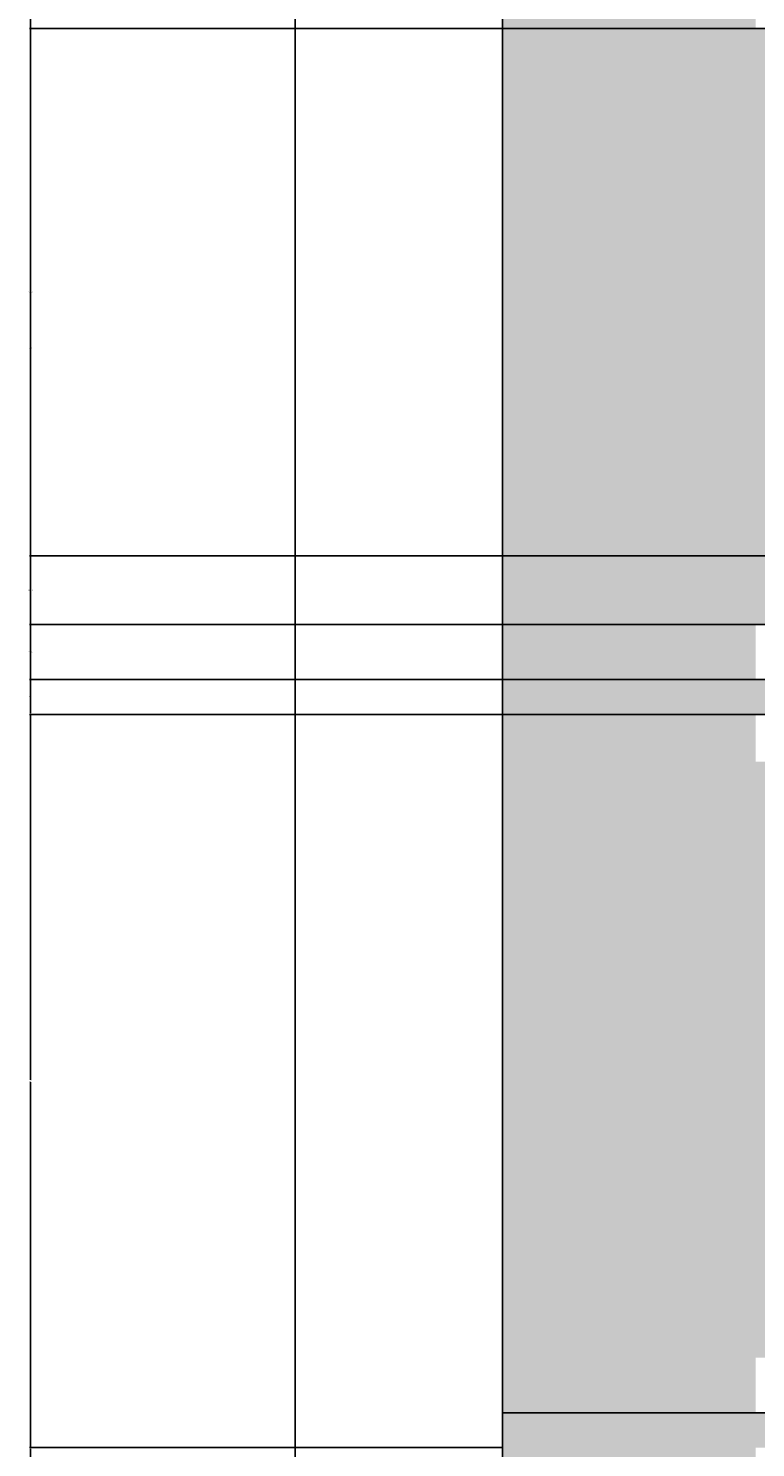
# Model space of a CAD drawing. Units: inches. Extents: x 3024 to 4744, y 1110 to 2100.
# Tile 18 of 29: x 3024 to 3149, y 1654 to 1897. Entities that reach past the tile are written whole.
import ezdxf

# ---------------------------------------------------------------- set-up
doc = ezdxf.new("R2010")
doc.units = ezdxf.units.IN
for name, color, linetype, lineweight in [('A-ANNO-DIMS', 2, 'Continuous', 18), ('A-ELEV', 7, 'Continuous', 25), ('A-ELEV-PATT', 252, 'Continuous', 13)]:
    doc.layers.add(name, color=color, linetype=linetype, lineweight=lineweight)
doc.styles.get("Standard").update_dxf_attribs({"font": 'arial.ttf'})
doc.dimstyles.get("Standard").update_dxf_attribs({"dimtxt": 0.18, "dimasz": 0.18, "dimexe": 0.18, "dimexo": 0.0625, "dimgap": 0.09, "dimtad": 0, "dimtih": 1, "dimtoh": 1, "dimdec": 1, "dimzin": 0, "dimdsep": 46, "dimlunit": 3, "dimtxsty": 'Standard', "dimcen": 0.09, "dimadec": 0, "dimazin": 0, "dimtfac": 1, "dimtdec": 1, "dimtofl": 0, "dimtmove": 0, "dimatfit": 3, "dimfxl": 1, "dimtolj": 1, "dimtzin": 0, "dimarcsym": 0})

# ---------------------------------------------------------------- blocks, each defined once
blk = doc.blocks.new('*D64')
at = {"layer": 'A-ANNO-DIMS', "color": 0, "lineweight": -2, "transparency": 16777216}
for p, q in [((3069.79, 1241.5), (3069.79, 2100.44)), ((3069.97, 2100.26), (3405.08, 2100.26)), ((3740.97, 2100.26), (3405.87, 2100.26)), ((3741.15, 1241.5), (3741.15, 2100.44))]:
    blk.add_line(p, q, dxfattribs=at)
at = {"layer": 'A-ANNO-DIMS', "color": 0, "transparency": 16777216}
for points in [[(3069.97, 2100.29), (3069.97, 2100.23), (3069.79, 2100.26)], [(3740.97, 2100.29), (3740.97, 2100.23), (3741.15, 2100.26)]]:
    blk.add_solid(points, dxfattribs=at)
at = {"layer": 'Defpoints', "color": 0, "transparency": 16777216}
for p in [(3741.15, 2100.26), (3069.79, 1241.43), (3741.15, 1241.43)]:
    blk.add_point(p, dxfattribs=at)
at = {"layer": 'A-ANNO-DIMS', "color": 0, "transparency": 16777216, "insert": (3405.47, 2100.26), "char_height": 0.18, "attachment_point": 5}
blk.add_mtext('\\A1;671.4', dxfattribs=at)
blk = doc.blocks.new('*D69')
at = {"layer": 'A-ANNO-DIMS', "color": 0, "lineweight": -2, "transparency": 16777216}
for p, q in [((3105.41, 1653.61), (3024.11, 1653.61)), ((3024.29, 1653.43), (3024.29, 1590.79)), ((3024.29, 1527.79), (3024.29, 1590.43)), ((3105.41, 1527.61), (3024.11, 1527.61))]:
    blk.add_line(p, q, dxfattribs=at)
at = {"layer": 'A-ANNO-DIMS', "color": 0, "transparency": 16777216}
for points in [[(3024.26, 1653.43), (3024.32, 1653.43), (3024.29, 1653.61)], [(3024.26, 1527.79), (3024.32, 1527.79), (3024.29, 1527.61)]]:
    blk.add_solid(points, dxfattribs=at)
at = {"layer": 'Defpoints', "color": 0, "transparency": 16777216}
for p in [(3024.29, 1653.61), (3105.47, 1653.61), (3105.47, 1527.61)]:
    blk.add_point(p, dxfattribs=at)
at = {"layer": 'A-ANNO-DIMS', "color": 0, "transparency": 16777216, "insert": (3024.29, 1590.61), "char_height": 0.18, "attachment_point": 5}
blk.add_mtext('\\A1;126', dxfattribs=at)
blk = doc.blocks.new('*D70')
at = {"layer": 'A-ANNO-DIMS', "color": 0, "lineweight": -2, "transparency": 16777216}
for p, q in [((3105.41, 1779.61), (3024.11, 1779.61)), ((3024.29, 1779.43), (3024.29, 1716.79)), ((3024.29, 1653.79), (3024.29, 1716.43)), ((3105.41, 1653.61), (3024.11, 1653.61))]:
    blk.add_line(p, q, dxfattribs=at)
at = {"layer": 'A-ANNO-DIMS', "color": 0, "transparency": 16777216}
for points in [[(3024.26, 1779.43), (3024.32, 1779.43), (3024.29, 1779.61)], [(3024.26, 1653.79), (3024.32, 1653.79), (3024.29, 1653.61)]]:
    blk.add_solid(points, dxfattribs=at)
at = {"layer": 'Defpoints', "color": 0, "transparency": 16777216}
for p in [(3024.29, 1779.61), (3105.47, 1779.61), (3105.47, 1653.61)]:
    blk.add_point(p, dxfattribs=at)
at = {"layer": 'A-ANNO-DIMS', "color": 0, "transparency": 16777216, "insert": (3024.29, 1716.61), "char_height": 0.18, "attachment_point": 5}
blk.add_mtext('\\A1;126', dxfattribs=at)
blk = doc.blocks.new('*D71')
at = {"layer": 'A-ANNO-DIMS', "color": 0, "lineweight": -2, "transparency": 16777216}
for p, q in [((3105.41, 1905.61), (3024.11, 1905.61)), ((3024.29, 1905.43), (3024.29, 1842.79)), ((3024.29, 1779.79), (3024.29, 1842.43)), ((3105.41, 1779.61), (3024.11, 1779.61))]:
    blk.add_line(p, q, dxfattribs=at)
at = {"layer": 'A-ANNO-DIMS', "color": 0, "transparency": 16777216}
for points in [[(3024.26, 1905.43), (3024.32, 1905.43), (3024.29, 1905.61)], [(3024.26, 1779.79), (3024.32, 1779.79), (3024.29, 1779.61)]]:
    blk.add_solid(points, dxfattribs=at)
at = {"layer": 'Defpoints', "color": 0, "transparency": 16777216}
for p in [(3024.29, 1905.61), (3105.47, 1905.61), (3105.47, 1779.61)]:
    blk.add_point(p, dxfattribs=at)
at = {"layer": 'A-ANNO-DIMS', "color": 0, "transparency": 16777216, "insert": (3024.29, 1842.61), "char_height": 0.18, "attachment_point": 5}
blk.add_mtext('\\A1;126', dxfattribs=at)
blk = doc.blocks.new('*D95')
at = {"layer": 'A-ANNO-DIMS', "color": 0, "lineweight": -2, "transparency": 16777216}
for p, q in [((3148.91, 1785.61), (3024.11, 1785.61)), ((3024.29, 1785.43), (3024.29, 1782.79)), ((3024.29, 1779.79), (3024.29, 1782.43)), ((3148.91, 1779.61), (3024.11, 1779.61))]:
    blk.add_line(p, q, dxfattribs=at)
at = {"layer": 'A-ANNO-DIMS', "color": 0, "transparency": 16777216}
for points in [[(3024.26, 1785.43), (3024.32, 1785.43), (3024.29, 1785.61)], [(3024.26, 1779.79), (3024.32, 1779.79), (3024.29, 1779.61)]]:
    blk.add_solid(points, dxfattribs=at)
at = {"layer": 'Defpoints', "color": 0, "transparency": 16777216}
for p in [(3024.29, 1785.61), (3148.97, 1785.61), (3148.97, 1779.61)]:
    blk.add_point(p, dxfattribs=at)
at = {"layer": 'A-ANNO-DIMS', "color": 0, "transparency": 16777216, "insert": (3024.29, 1782.61), "char_height": 0.18, "attachment_point": 5}
blk.add_mtext('\\A1;6.00', dxfattribs=at)
blk = doc.blocks.new('*D96')
at = {"layer": 'A-ANNO-DIMS', "color": 0, "lineweight": -2, "transparency": 16777216}
for p, q in [((3148.91, 1795.04), (3024.11, 1795.04)), ((3024.29, 1794.86), (3024.29, 1790.51)), ((3024.29, 1785.79), (3024.29, 1790.15)), ((3148.91, 1785.61), (3024.11, 1785.61))]:
    blk.add_line(p, q, dxfattribs=at)
at = {"layer": 'A-ANNO-DIMS', "color": 0, "transparency": 16777216}
for points in [[(3024.26, 1794.86), (3024.32, 1794.86), (3024.29, 1795.04)], [(3024.26, 1785.79), (3024.32, 1785.79), (3024.29, 1785.61)]]:
    blk.add_solid(points, dxfattribs=at)
at = {"layer": 'Defpoints', "color": 0, "transparency": 16777216}
for p in [(3024.29, 1795.04), (3148.97, 1795.04), (3148.97, 1785.61)]:
    blk.add_point(p, dxfattribs=at)
at = {"layer": 'A-ANNO-DIMS', "color": 0, "transparency": 16777216, "insert": (3024.29, 1790.33), "char_height": 0.18, "attachment_point": 5}
blk.add_mtext('\\A1;9.432', dxfattribs=at)
blk = doc.blocks.new('*D97')
at = {"layer": 'A-ANNO-DIMS', "color": 0, "lineweight": -2, "transparency": 16777216}
for p, q in [((3151.6, 1806.87), (3024.11, 1806.87)), ((3024.29, 1806.69), (3024.29, 1801.14)), ((3024.29, 1795.22), (3024.29, 1800.77)), ((3151.6, 1795.04), (3024.11, 1795.04))]:
    blk.add_line(p, q, dxfattribs=at)
at = {"layer": 'A-ANNO-DIMS', "color": 0, "transparency": 16777216}
for points in [[(3024.26, 1806.69), (3024.32, 1806.69), (3024.29, 1806.87)], [(3024.26, 1795.22), (3024.32, 1795.22), (3024.29, 1795.04)]]:
    blk.add_solid(points, dxfattribs=at)
at = {"layer": 'Defpoints', "color": 0, "transparency": 16777216}
for p in [(3024.29, 1806.87), (3151.66, 1806.87), (3151.66, 1795.04)]:
    blk.add_point(p, dxfattribs=at)
at = {"layer": 'A-ANNO-DIMS', "color": 0, "transparency": 16777216, "insert": (3024.29, 1800.96), "char_height": 0.18, "attachment_point": 5}
blk.add_mtext('\\A1;11.824', dxfattribs=at)
blk = doc.blocks.new('*D98')
at = {"layer": 'A-ANNO-DIMS', "color": 0, "lineweight": -2, "transparency": 16777216}
for p, q in [((3154.27, 1897.49), (3024.11, 1897.49)), ((3024.29, 1897.31), (3024.29, 1852.36)), ((3024.29, 1807.05), (3024.29, 1852)), ((3154.27, 1806.87), (3024.11, 1806.87))]:
    blk.add_line(p, q, dxfattribs=at)
at = {"layer": 'A-ANNO-DIMS', "color": 0, "transparency": 16777216}
for points in [[(3024.26, 1897.31), (3024.32, 1897.31), (3024.29, 1897.49)], [(3024.26, 1807.05), (3024.32, 1807.05), (3024.29, 1806.87)]]:
    blk.add_solid(points, dxfattribs=at)
at = {"layer": 'Defpoints', "color": 0, "transparency": 16777216}
for p in [(3024.29, 1897.49), (3154.33, 1897.49), (3154.33, 1806.87)]:
    blk.add_point(p, dxfattribs=at)
at = {"layer": 'A-ANNO-DIMS', "color": 0, "transparency": 16777216, "insert": (3024.29, 1852.18), "char_height": 0.18, "attachment_point": 5}
blk.add_mtext('\\A1;90.62', dxfattribs=at)

msp = doc.modelspace()

# ---------------------------------------------------------------- hatches: boundary and pattern name
at = {"layer": 'A-ELEV-PATT'}
h = msp.add_hatch(color=256, dxfattribs=at)
h.dxf.hatch_style = 1
h.paths.add_polyline_path([(3329.7033, 1407.6112), (3105.4722, 1407.6112), (3105.4722, 1401.6112), (3329.7033, 1401.6112)])
h.paths.add_polyline_path([(3329.7033, 1281.6112), (3105.4722, 1281.6112), (3105.4722, 1275.6112), (3112.3838, 1275.6112), (3329.7033, 1275.6112)])
h.paths.add_polyline_path([(3329.7033, 1533.6112), (3105.4722, 1533.6112), (3105.4722, 1527.6112), (3329.7033, 1527.6112)])
h.paths.add_polyline_path([(3329.7033, 1659.6112), (3105.4722, 1659.6112), (3105.4722, 1653.6112), (3329.7033, 1653.6112)])
h.paths.add_polyline_path([(3329.7033, 1785.6112), (3105.4722, 1785.6112), (3105.4722, 1779.6112), (3329.7033, 1779.6112)])
h.paths.add_polyline_path([(3329.7033, 1911.6112), (3105.4722, 1911.6112), (3095.7158, 1911.6112), (3095.7158, 1905.6112), (3329.7033, 1905.6112)])
h.paths.add_polyline_path([(3715.2286, 1911.6112), (3705.4722, 1911.6112), (3705.4722, 1905.6112), (3715.2286, 1905.6112)])
h.paths.add_polyline_path([(3688.5588, 1911.6112), (3481.2411, 1911.6112), (3481.2411, 1905.6112), (3688.5588, 1905.6112)])
h = msp.add_hatch(color=256, dxfattribs=at)
h.dxf.hatch_style = 1
h.paths.add_polyline_path([(3154.3287, 1897.4879), (3148.9694, 1897.4879), (3148.9694, 1905.6112), (3105.4722, 1905.6112), (3105.4722, 1785.6112), (3148.9694, 1785.6112), (3148.9694, 1795.0431), (3151.6604, 1795.0431), (3151.6604, 1806.8674), (3154.3287, 1806.8674)])
h.paths.add_polyline_path([(3329.7033, 1905.6112), (3292.6051, 1905.6112), (3292.6051, 1897.4879), (3287.2458, 1897.4879), (3287.2458, 1806.8674), (3288.3759, 1806.8674), (3288.3759, 1795.0431), (3292.6051, 1795.0431), (3292.6051, 1785.6112), (3329.7033, 1785.6112)])
h.paths.add_polyline_path([(3154.3287, 1771.4879), (3148.9694, 1771.4879), (3148.9694, 1779.6112), (3105.4722, 1779.6112), (3105.4722, 1659.6112), (3148.9694, 1659.6112), (3148.9694, 1669.0431), (3151.6604, 1669.0431), (3151.6604, 1680.8674), (3154.3287, 1680.8674)])
h.paths.add_polyline_path([(3329.7033, 1779.6112), (3292.6051, 1779.6112), (3292.6051, 1771.4879), (3287.2458, 1771.4879), (3287.2458, 1680.8674), (3288.3759, 1680.8674), (3288.3759, 1669.0431), (3292.6051, 1669.0431), (3292.6051, 1659.6112), (3329.7033, 1659.6112)])
h.paths.add_polyline_path([(3154.3287, 1645.4879), (3148.9694, 1645.4879), (3148.9694, 1653.6112), (3105.4722, 1653.6112), (3105.4722, 1533.6112), (3148.9694, 1533.6112), (3148.9694, 1543.0431), (3151.6604, 1543.0431), (3151.6604, 1554.8674), (3154.3287, 1554.8674)])
h.paths.add_polyline_path([(3329.7033, 1653.6112), (3292.6051, 1653.6112), (3292.6051, 1645.4879), (3287.2458, 1645.4879), (3287.2458, 1554.8674), (3288.3759, 1554.8674), (3288.3759, 1543.0431), (3292.6051, 1543.0431), (3292.6051, 1533.6112), (3329.7033, 1533.6112)])
h.paths.add_polyline_path([(3329.7033, 1527.6112), (3292.6051, 1527.6112), (3292.6051, 1519.4879), (3287.2458, 1519.4879), (3287.2458, 1428.8674), (3288.3759, 1428.8674), (3288.3759, 1417.0431), (3292.6051, 1417.0431), (3292.6051, 1407.6112), (3329.7033, 1407.6112)])
h.paths.add_polyline_path([(3329.7033, 1401.6112), (3292.6051, 1401.6112), (3292.6051, 1393.4879), (3287.2458, 1393.4879), (3287.2458, 1302.8674), (3288.3759, 1302.8674), (3288.3759, 1291.0431), (3292.6051, 1291.0431), (3292.6051, 1281.6112), (3329.7033, 1281.6112)])
h.paths.add_polyline_path([(3154.3287, 1393.4879), (3148.9694, 1393.4879), (3148.9694, 1401.6112), (3105.4722, 1401.6112), (3105.4722, 1281.6112), (3148.9694, 1281.6112), (3148.9694, 1291.0431), (3151.6604, 1291.0431), (3151.6604, 1302.8674), (3154.3287, 1302.8674)])
h.paths.add_polyline_path([(3154.3287, 1519.4879), (3148.9694, 1519.4879), (3148.9694, 1527.6112), (3105.4722, 1527.6112), (3105.4722, 1407.6112), (3148.9694, 1407.6112), (3148.9694, 1417.0431), (3151.6604, 1417.0431), (3151.6604, 1428.8674), (3154.3287, 1428.8674)])
h.paths.add_polyline_path([(3515.7606, 1897.4879), (3510.4013, 1897.4879), (3510.4013, 1905.6112), (3481.2411, 1905.6112), (3481.2411, 1785.6112), (3510.4013, 1785.6112), (3510.4013, 1795.0431), (3513.0923, 1795.0431), (3513.0923, 1806.8674), (3515.7606, 1806.8674)])
h.paths.add_polyline_path([(3688.5588, 1905.6112), (3654.037, 1905.6112), (3654.037, 1897.4879), (3648.6777, 1897.4879), (3648.6777, 1806.8674), (3649.8078, 1806.8674), (3649.8078, 1795.0431), (3654.037, 1795.0431), (3654.037, 1785.6112), (3688.5588, 1785.6112)])
h.paths.add_polyline_path([(3515.7606, 1771.4879), (3510.4013, 1771.4879), (3510.4013, 1779.6112), (3481.2411, 1779.6112), (3481.2411, 1659.6112), (3510.4013, 1659.6112), (3510.4013, 1669.0431), (3513.0923, 1669.0431), (3513.0923, 1680.8674), (3515.7606, 1680.8674)])
h.paths.add_polyline_path([(3688.5588, 1779.6112), (3654.037, 1779.6112), (3654.037, 1771.4879), (3648.6777, 1771.4879), (3648.6777, 1680.8674), (3649.8078, 1680.8674), (3649.8078, 1669.0431), (3654.037, 1669.0431), (3654.037, 1659.6112), (3688.5588, 1659.6112)])
h.paths.add_polyline_path([(3515.7606, 1645.4879), (3510.4013, 1645.4879), (3510.4013, 1653.6112), (3481.2411, 1653.6112), (3481.2411, 1533.6112), (3510.4013, 1533.6112), (3510.4013, 1543.0431), (3513.0923, 1543.0431), (3513.0923, 1554.8674), (3515.7606, 1554.8674)])
h.paths.add_polyline_path([(3688.5588, 1653.6112), (3654.037, 1653.6112), (3654.037, 1645.4879), (3648.6777, 1645.4879), (3648.6777, 1554.8674), (3649.8078, 1554.8674), (3649.8078, 1543.0431), (3654.037, 1543.0431), (3654.037, 1533.6112), (3688.5588, 1533.6112)])
h.paths.add_polyline_path([(3515.7606, 1519.4879), (3510.4013, 1519.4879), (3510.4013, 1527.6112), (3481.2411, 1527.6112), (3481.2411, 1407.6112), (3510.4013, 1407.6112), (3510.4013, 1417.0431), (3513.0923, 1417.0431), (3513.0923, 1428.8674), (3515.7606, 1428.8674)])
h.paths.add_polyline_path([(3688.5588, 1527.6112), (3654.037, 1527.6112), (3654.037, 1519.4879), (3648.6777, 1519.4879), (3648.6777, 1428.8674), (3649.8078, 1428.8674), (3649.8078, 1417.0431), (3654.037, 1417.0431), (3654.037, 1407.6112), (3688.5588, 1407.6112)])
h.paths.add_polyline_path([(3515.7606, 1393.4879), (3510.4013, 1393.4879), (3510.4013, 1401.6112), (3481.2411, 1401.6112), (3481.2411, 1281.6112), (3510.4013, 1281.6112), (3510.4013, 1291.0431), (3513.0923, 1291.0431), (3513.0923, 1302.8674), (3515.7606, 1302.8674)])
h.paths.add_polyline_path([(3688.5588, 1401.6112), (3654.037, 1401.6112), (3654.037, 1393.4879), (3648.6777, 1393.4879), (3648.6777, 1302.8674), (3649.8078, 1302.8674), (3649.8078, 1291.0431), (3654.037, 1291.0431), (3654.037, 1281.6112), (3688.5588, 1281.6112)])
h.paths.add_polyline_path([(3515.7606, 1267.4879), (3510.4013, 1267.4879), (3510.4013, 1275.6112), (3481.2411, 1275.6112), (3481.2411, 1155.6112), (3510.4013, 1155.6112), (3510.4013, 1165.0431), (3513.0923, 1165.0431), (3513.0923, 1176.8674), (3515.7606, 1176.8674)])
h.paths.add_polyline_path([(3688.5588, 1275.6112), (3654.037, 1275.6112), (3654.037, 1267.4879), (3648.6777, 1267.4879), (3648.6777, 1176.8674), (3649.8078, 1176.8674), (3649.8078, 1165.0431), (3654.037, 1165.0431), (3654.037, 1155.6112), (3688.5588, 1155.6112)])
h.paths.add_polyline_path([(3112.3838, 1275.6112), (3105.4722, 1275.6112), (3105.4722, 1171.0239), (3112.3838, 1171.0239)])

# ---------------------------------------------------------------- linework, layer by layer
at = {"layer": 'A-ELEV'}
for p, q in [((3105.4722, 1171.0239), (3105.4722, 1905.6112)), ((3105.4722, 1171.0239), (3105.4722, 1905.6112)), ((3105.4722, 1785.6112), (3329.7033, 1785.6112)), ((3105.4722, 1785.6112), (3329.7033, 1785.6112)), ((3329.7033, 1779.6112), (3105.4722, 1779.6112)), ((3329.7033, 1779.6112), (3105.4722, 1779.6112)), ((3105.4722, 1659.6112), (3329.7033, 1659.6112)), ((3105.4722, 1659.6112), (3329.7033, 1659.6112))]:
    msp.add_line(p, q, dxfattribs=at)

# ---------------------------------------------------------------- dimensions: what is measured, and where the dimension line sits
at = {"layer": 'A-ANNO-DIMS'}
dim = msp.add_linear_dim(base=(3741.1507, 2100.2584), p1=(3069.7937, 1241.4341), p2=(3741.1507, 1241.4341), dimstyle='Standard', override={"dimdec": 1, "dimlfac": 1, "dimrnd": 0, "dimzin": 0, "dimdsep": 46, "dimlunit": 2}, dxfattribs=at)
dim.commit()
dim.dimension.update_dxf_attribs({"geometry": '*D64', "text_midpoint": (3405.4722, 2100.2584)})
for base, p1, p2, override, picture, middle in [((3024.2937, 1905.6112), (3105.4722, 1779.6112), (3105.4722, 1905.6112), {"dimdec": 0, "dimlfac": 1, "dimrnd": 0, "dimzin": 0, "dimdsep": 46, "dimlunit": 2}, '*D71', (3024.2937, 1842.6112)), ((3024.2937, 1897.4879), (3154.3287, 1806.8674), (3154.3287, 1897.4879), {"dimdec": 2, "dimlfac": 1, "dimrnd": 0, "dimzin": 0, "dimdsep": 46, "dimlunit": 2}, '*D98', (3024.2937, 1852.1776)), ((3024.2937, 1806.8674), (3151.6604, 1795.0431), (3151.6604, 1806.8674), {"dimdec": 3, "dimlfac": 1, "dimrnd": 0, "dimzin": 0, "dimdsep": 46, "dimlunit": 2}, '*D97', (3024.2937, 1800.9553)), ((3024.2937, 1795.0431), (3148.9694, 1785.6112), (3148.9694, 1795.0431), {"dimdec": 3, "dimlfac": 1, "dimrnd": 0, "dimzin": 0, "dimdsep": 46, "dimlunit": 2}, '*D96', (3024.2937, 1790.3271)), ((3024.2937, 1785.6112), (3148.9694, 1779.6112), (3148.9694, 1785.6112), {"dimdec": 2, "dimlfac": 1, "dimrnd": 0, "dimzin": 0, "dimdsep": 46, "dimlunit": 2}, '*D95', (3024.2937, 1782.6112)), ((3024.2937, 1779.6112), (3105.4722, 1653.6112), (3105.4722, 1779.6112), {"dimdec": 0, "dimlfac": 1, "dimrnd": 0, "dimzin": 0, "dimdsep": 46, "dimlunit": 2}, '*D70', (3024.2937, 1716.6112)), ((3024.2937, 1653.6112), (3105.4722, 1527.6112), (3105.4722, 1653.6112), {"dimdec": 0, "dimlfac": 1, "dimrnd": 0, "dimzin": 0, "dimdsep": 46, "dimlunit": 2}, '*D69', (3024.2937, 1590.6112))]:
    dim = msp.add_linear_dim(base=base, p1=p1, p2=p2, angle=90, dimstyle='Standard', override=override, dxfattribs=at)
    dim.commit()
    dim.dimension.update_dxf_attribs({"geometry": picture, "text_midpoint": middle})

doc.saveas('drawing.dxf')
